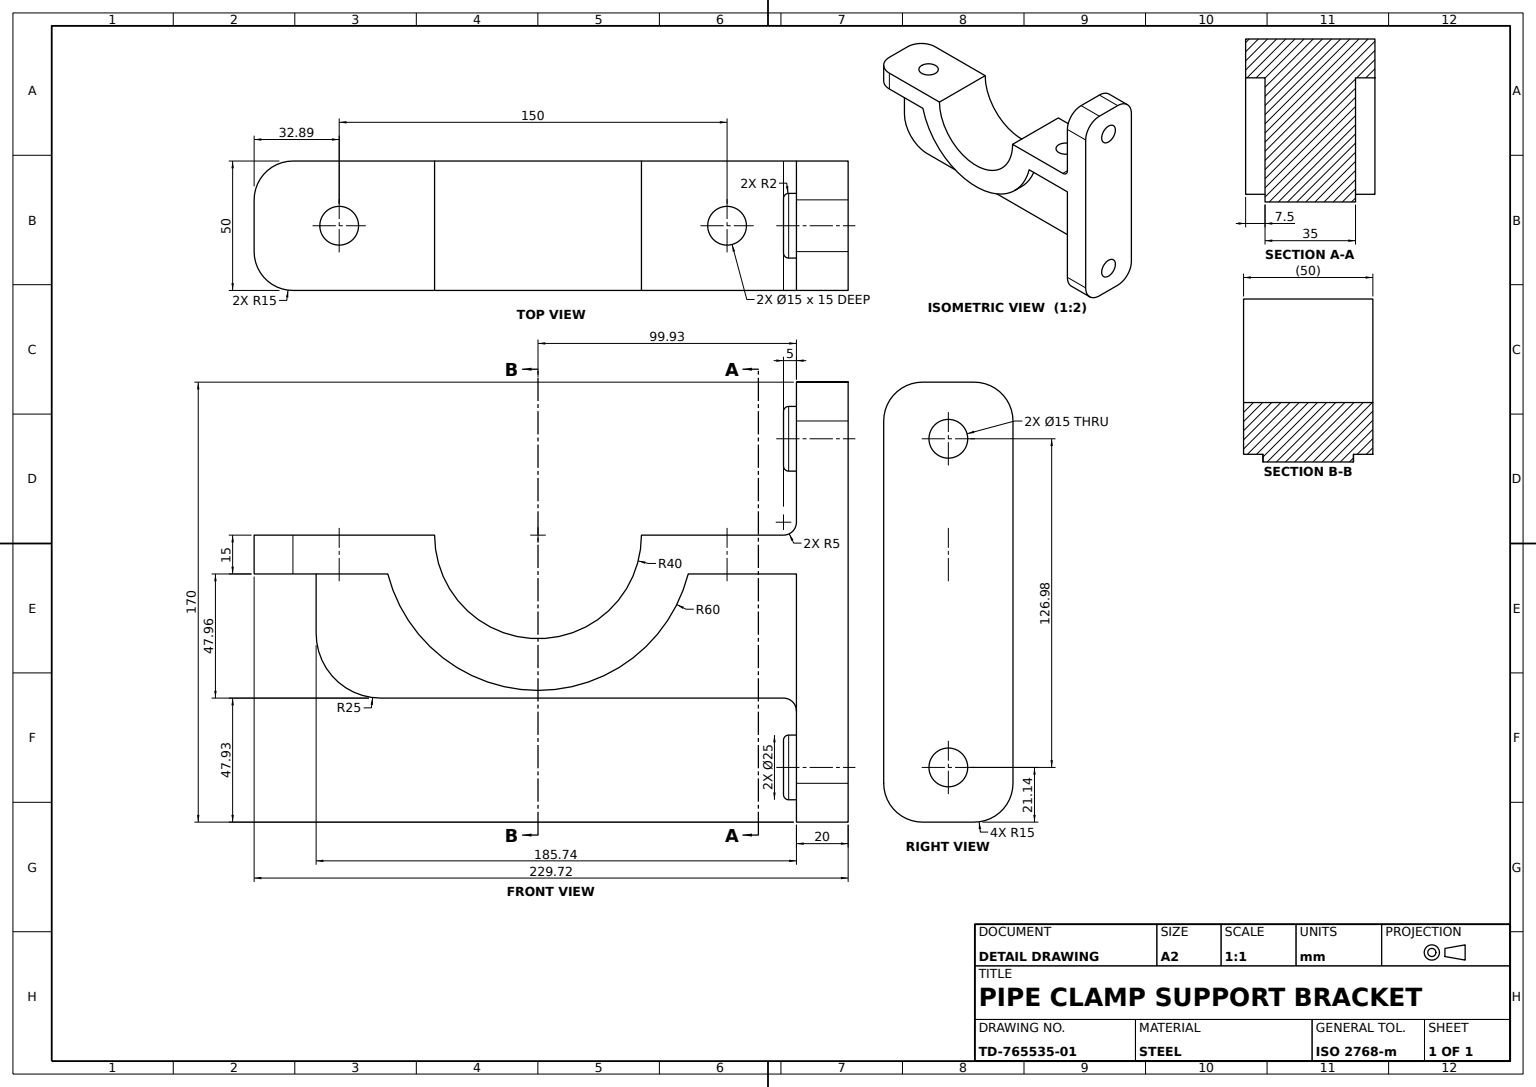
SolidWorks part; units mm, degrees
material "Plain Carbon Steel"
ref_plane "Front Plane" through (0, 0, 0) normal (0, 0, 1) x (1, 0, 0)
ref_plane "Top Plane" through (0, 0, 0) normal (0, 1, 0) x (1, 0, 0)
ref_plane "Right Plane" through (0, 0, 0) normal (1, 0, 0) x (0, 0, -1)
sketch "Base Plate Sketch" plane through (0, 0, 0) normal (0, 0, 1) x (1, 0, 0)
  line L1 (-25, 85) -> (25, 85)
  line L2 (-25, 85) -> (-25, -85)
  line L3 (-25, -85) -> (25, -85)
  line L4 (25, 85) -> (25, -85)
  line L5 (-25, 85) -> (25, -85) construction
  line L6 (-25, -85) -> (25, 85) construction
  point P0 (0, 0)
  dimension "D1" = 170
  dimension "D2" = 50
extrude "Base Plate 170x50x20" add sketch "Base Plate Sketch" along normal blind 20
sketch "Clamp Saddle Sketch" plane through (0, 0, 0) normal (1, 0, 0) x (0, 0, -1)
  line L9 (-159.9345, 25.89) -> (-179.9345, 25.89)
  line L10 (-79.9345, 25.89) -> (-20, 25.89)
  line L15 (-61.8397, 10.89) -> (-20, 10.89)
  line L18 (-20, 10.89) -> (-20, 25.89)
  line L20 (-20, -85) -> (-20, 85) construction
  line L21 (-179.9345, 25.89) -> (-229.7176, 25.89)
  line L24 (-229.7176, 10.89) -> (-229.7176, 25.89)
  line L25 (-178.0292, 10.89) -> (-229.7176, 10.89)
  arc A6 (-178.0292, 10.89) -> (-61.8397, 10.89) centre (-119.9345, 25.89) ccw
  arc A7 (-159.9345, 25.89) -> (-79.9345, 25.89) centre (-119.9345, 25.89) ccw
  dimension "D1" = 120
  dimension "D2" = 80
  dimension "D3" = 15
  dimension "D4" = 10.89
  dimension "D5" = 99.9345
  dimension "D6" = 20
  dimension "D7" = 49.7831
extrude "Clamp Saddle" add sketch "Clamp Saddle Sketch" along normal mid plane 50 contours A6 L15 L18 L10 A7 L9 L21 L24 L25
fillet "Saddle Fillet R15" radius 15 2 edges at (-25, 18.39, 229.7176) (25, 18.39, 229.7176)
fillet "Saddle To Plate Fillet R5" radius 5 1 edges at (0, 25.89, 20)
sketch "Clamp Bolt Holes Sketch" plane through (0, 25.89, 0) normal (0, 1, 0) x (1, 0, 0)
  line L0 (-25, -159.9345) -> (-25, -214.7176) construction
  circle A0 centre (0, -46.8227) radius 7.5
  circle A1 centre (0, -196.8227) radius 7.5
  dimension "D2" = 15
  dimension "D3" = 15
  dimension "D1" = 150
  dimension "D4" = 25
  dimension "D5" = 32.8949
extrude "Clamp Bolt Holes 2xØ15" cut sketch "Clamp Bolt Holes Sketch" against normal mid plane 50
sketch "Mounting Holes Sketch" plane through (0, 0, 20) normal (0, 0, 1) x (1, 0, 0)
  line L0 (-25, 85) -> (-25, 30.89) construction
  line L1 (-25, 30.89) -> (25, 30.89) construction
  circle A0 centre (0, 63.1222) radius 7.5
  circle A1 centre (0, -63.8619) radius 7.5
  dimension "D1" = 15
  dimension "D2" = 15
  dimension "D3" = 25
  dimension "D4" = 32.2322
  dimension "D5" = 94.7519
extrude "Mounting Holes 2xØ15" cut sketch "Mounting Holes Sketch" against normal mid plane 50
sketch "Mounting Hole Bosses Sketch" plane through (0, 0, 20) normal (0, 0, 1) x (1, 0, 0)
  circle A0 centre (0, 63.1222) radius 12.5
  circle A1 centre (0, -63.8619) radius 12.5
  circle A2 centre (0, -63.8619) radius 7.5 construction
  circle A3 centre (0, -63.8619) radius 7.5
  circle A4 centre (0, 63.1222) radius 7.5 construction
  circle A5 centre (0, 63.1222) radius 7.5
  dimension "D1" = 25
  dimension "D2" = 25
extrude "Mounting Hole Bosses Ø25" add sketch "Mounting Hole Bosses Sketch" along normal blind 5
fillet "Hole Boss Fillet R2" radius 2 2 edges at (12.5, -63.8619, 25) (12.5, 63.1222, 25)
fillet "Base Plate Corner Fillets R15" radius 15 4 edges at (-25, 85, 10) (-25, -85, 10) (25, -85, 10) (25, 85, 10)
sketch "Support Rib Sketch" plane through (0, 0, 0) normal (1, 0, 0) x (0, 0, -1)
  line L0 (-20, -70) -> (-20, 10.89) construction
  line L2 (-205.743, 10.89) -> (-205.743, -37.0746)
  line L3 (-205.743, -37.0746) -> (-20, -37.0746)
  line L4 (-20, 10.89) -> (-20, -37.0746)
  line L5 (-61.8397, 10.89) -> (-20, 10.89) construction
  line L6 (-178.0292, 10.89) -> (-214.7176, 10.89) construction
  line L7 (-61.8397, 10.89) -> (-20, 10.89)
  line L8 (-178.0292, 10.89) -> (-205.743, 10.89)
  arc A0 (-178.0292, 10.89) -> (-61.8397, 10.89) centre (-119.9345, 25.89) ccw construction
  arc A1 (-178.0292, 10.89) -> (-61.8397, 10.89) centre (-119.9345, 25.89) ccw
  dimension "D1" = 185.743
  dimension "D2" = 47.9646
extrude "Support Rib" add sketch "Support Rib Sketch" along normal mid plane 35
fillet "Support Rib Fillet R25" radius 25 1 edges at (0, -37.0746, 205.743)
fillet "Rib To Plate Fillet R5" radius 5 1 edges at (0, -37.0746, 20)
